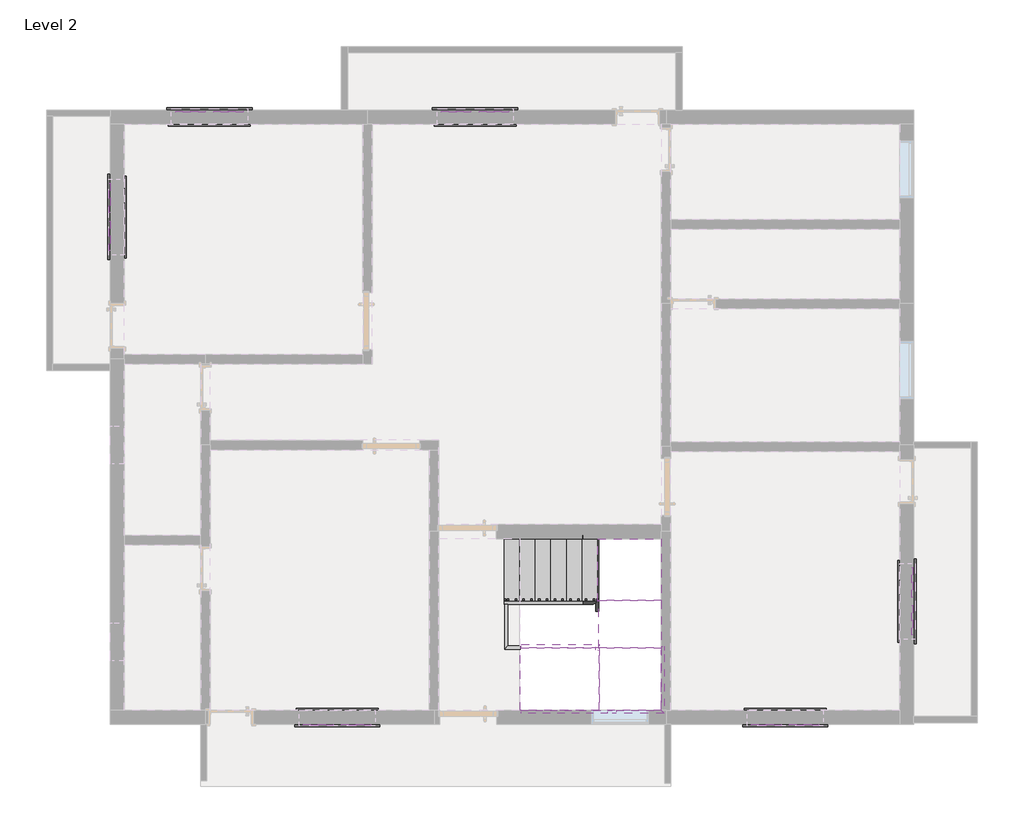
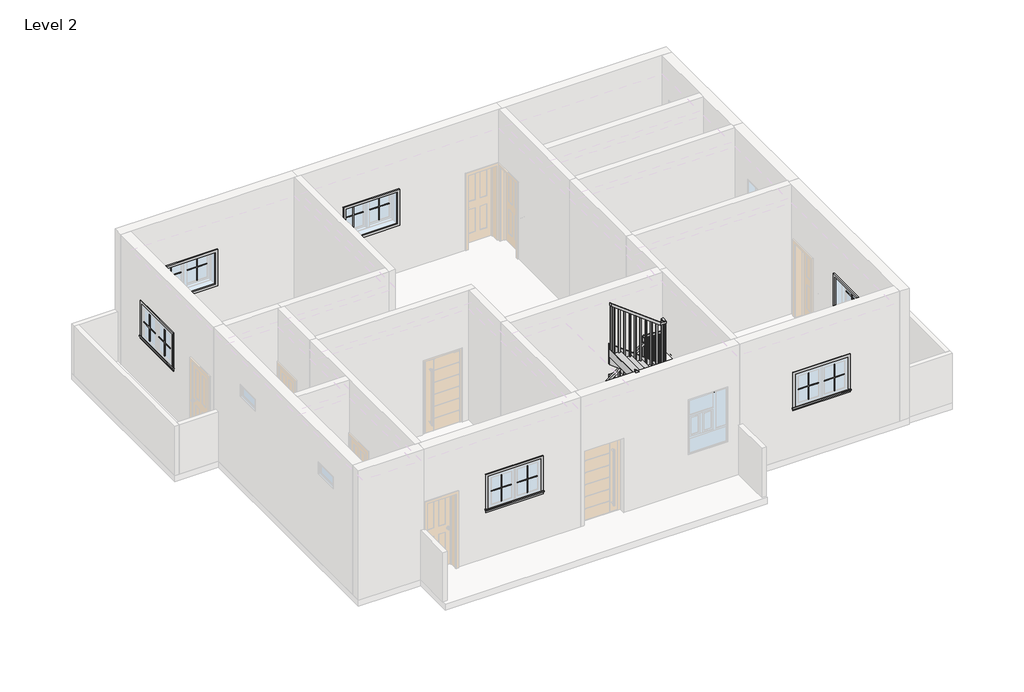
# One storey, part 3 of 3: 24 proxies, 11 members, 3 stair flights, 2 railings, 2 slabs.
"""IFC4 building model written with IfcOpenShell, lengths in millimetres."""

from ifc_helpers import new_model, si_unit, frame, origin, place, context, project, spatial, polyline, outline, extrude, faceted_brep, transform, mapped, element, save
from components import m_muntin_pattern_2x2_m_muntin_pattern_2x2_8d9e5da3, m_muntin_pattern_2x2_m_muntin_pattern_2x2_32a0f80e, m_trim_window_exterior_flat_with_sill_3a557199, m_trim_window_interior_flat_picture_frame_580345df, non_monolithic_landing_c08c66cc, non_monolithic_landing_bd582a30, stair_flight_50mm_tread_13mm_riser_0f073b0c, stair_flight_50mm_tread_13mm_riser_a88b1a6b, stair_flight_50mm_tread_13mm_riser_70c7a40c

model = new_model("IFC4")

# Units and contexts
model_context = context("Model", 3, world=origin())
ifc_project = project(units=[si_unit("LENGTHUNIT", "METRE", prefix="MILLI")], contexts=[model_context])

# Site, building, storey
site = spatial("IfcSite", under=ifc_project)
building = spatial("IfcBuilding", under=site)
storey = spatial("IfcBuildingStorey", under=building, Name="Level 2", Elevation=3200.4)

# Proxies
placement = place(None, origin())
m_muntin_pattern_2x2_m_muntin_pattern_2x2_shape = m_muntin_pattern_2x2_m_muntin_pattern_2x2_8d9e5da3(model_context)
element("IfcBuildingElementProxy", 1, Name="M_Muntin Pattern_2x2 : M_Muntin Pattern_2x2", ObjectType="M_Muntin Pattern_2x2 : M_Muntin Pattern_2x2", at=placement, inside=storey, context=model_context, shape_type="MappedRepresentation", body=[
    mapped(m_muntin_pattern_2x2_m_muntin_pattern_2x2_shape, transform((-14356.7669909, -4470.2368509, 4489.45), x_axis=(-1.0, 0.0, 0.0), y_axis=(0.0, -1.0, 0.0), z_axis=(0.0, 0.0, 1.0))),
])
element("IfcBuildingElementProxy", 2, Name="M_Muntin Pattern_2x2 : M_Muntin Pattern_2x2", ObjectType="M_Muntin Pattern_2x2 : M_Muntin Pattern_2x2", at=placement, inside=storey, context=model_context, shape_type="MappedRepresentation", body=[
    mapped(m_muntin_pattern_2x2_m_muntin_pattern_2x2_shape, transform((-17007.0919909, 5340.5131491, 4489.45), x_axis=(1.0, 0.0, 0.0), y_axis=(0.0, 1.0, 0.0), z_axis=(0.0, 0.0, 1.0))),
])
element("IfcBuildingElementProxy", 3, Name="M_Muntin Pattern_2x2 : M_Muntin Pattern_2x2", ObjectType="M_Muntin Pattern_2x2 : M_Muntin Pattern_2x2", at=placement, inside=storey, context=model_context, shape_type="MappedRepresentation", body=[
    mapped(m_muntin_pattern_2x2_m_muntin_pattern_2x2_shape, transform((-18281.8544909, 3334.7006491, 4489.45), x_axis=(0.0, 1.0, 0.0), y_axis=(-1.0, 0.0, 0.0), z_axis=(0.0, 0.0, 1.0))),
])
element("IfcBuildingElementProxy", 4, Name="M_Muntin Pattern_2x2 : M_Muntin Pattern_2x2", ObjectType="M_Muntin Pattern_2x2 : M_Muntin Pattern_2x2", at=placement, inside=storey, context=model_context, shape_type="MappedRepresentation", body=[
    mapped(m_muntin_pattern_2x2_m_muntin_pattern_2x2_shape, transform((-12757.3544909, 5340.5131491, 4489.45), x_axis=(1.0, 0.0, 0.0), y_axis=(0.0, 1.0, 0.0), z_axis=(0.0, 0.0, 1.0))),
])
element("IfcBuildingElementProxy", 5, Name="M_Muntin Pattern_2x2 : M_Muntin Pattern_2x2", ObjectType="M_Muntin Pattern_2x2 : M_Muntin Pattern_2x2", at=placement, inside=storey, context=model_context, shape_type="MappedRepresentation", body=[
    mapped(m_muntin_pattern_2x2_m_muntin_pattern_2x2_shape, transform((-5448.5044909, -2207.2493509, 4489.45), x_axis=(0.0, -1.0, 0.0), y_axis=(1.0, 0.0, 0.0), z_axis=(0.0, 0.0, 1.0))),
])
element("IfcBuildingElementProxy", 6, Name="M_Muntin Pattern_2x2 : M_Muntin Pattern_2x2", ObjectType="M_Muntin Pattern_2x2 : M_Muntin Pattern_2x2", at=placement, inside=storey, context=model_context, shape_type="MappedRepresentation", body=[
    mapped(m_muntin_pattern_2x2_m_muntin_pattern_2x2_shape, transform((-7193.1669909, -4470.2368509, 4489.45), x_axis=(-1.0, 0.0, 0.0), y_axis=(0.0, -1.0, 0.0), z_axis=(0.0, 0.0, 1.0))),
])
m_muntin_pattern_2x2_m_muntin_pattern_2x2_2_shape = m_muntin_pattern_2x2_m_muntin_pattern_2x2_32a0f80e(model_context)
element("IfcBuildingElementProxy", 7, Name="M_Muntin Pattern_2x2 : M_Muntin Pattern_2x2", ObjectType="M_Muntin Pattern_2x2 : M_Muntin Pattern_2x2", at=placement, inside=storey, context=model_context, shape_type="MappedRepresentation", body=[
    mapped(m_muntin_pattern_2x2_m_muntin_pattern_2x2_2_shape, transform((-14963.1919909, -4470.2368509, 4489.45), x_axis=(1.0, 0.0, 0.0), y_axis=(0.0, 1.0, 0.0), z_axis=(0.0, 0.0, 1.0))),
])
element("IfcBuildingElementProxy", 8, Name="M_Muntin Pattern_2x2 : M_Muntin Pattern_2x2", ObjectType="M_Muntin Pattern_2x2 : M_Muntin Pattern_2x2", at=placement, inside=storey, context=model_context, shape_type="MappedRepresentation", body=[
    mapped(m_muntin_pattern_2x2_m_muntin_pattern_2x2_2_shape, transform((-16400.6669909, 5340.5131491, 4489.45), x_axis=(-1.0, 0.0, 0.0), y_axis=(0.0, -1.0, 0.0), z_axis=(0.0, 0.0, 1.0))),
])
element("IfcBuildingElementProxy", 9, Name="M_Muntin Pattern_2x2 : M_Muntin Pattern_2x2", ObjectType="M_Muntin Pattern_2x2 : M_Muntin Pattern_2x2", at=placement, inside=storey, context=model_context, shape_type="MappedRepresentation", body=[
    mapped(m_muntin_pattern_2x2_m_muntin_pattern_2x2_2_shape, transform((-18281.8544909, 3941.1256491, 4489.45), x_axis=(0.0, -1.0, 0.0), y_axis=(1.0, 0.0, 0.0), z_axis=(0.0, 0.0, 1.0))),
])
element("IfcBuildingElementProxy", 10, Name="M_Muntin Pattern_2x2 : M_Muntin Pattern_2x2", ObjectType="M_Muntin Pattern_2x2 : M_Muntin Pattern_2x2", at=placement, inside=storey, context=model_context, shape_type="MappedRepresentation", body=[
    mapped(m_muntin_pattern_2x2_m_muntin_pattern_2x2_2_shape, transform((-12150.9294909, 5340.5131491, 4489.45), x_axis=(-1.0, 0.0, 0.0), y_axis=(0.0, -1.0, 0.0), z_axis=(0.0, 0.0, 1.0))),
])
element("IfcBuildingElementProxy", 11, Name="M_Muntin Pattern_2x2 : M_Muntin Pattern_2x2", ObjectType="M_Muntin Pattern_2x2 : M_Muntin Pattern_2x2", at=placement, inside=storey, context=model_context, shape_type="MappedRepresentation", body=[
    mapped(m_muntin_pattern_2x2_m_muntin_pattern_2x2_2_shape, transform((-5448.5044909, -2813.6743509, 4489.45), x_axis=(0.0, 1.0, 0.0), y_axis=(-1.0, 0.0, 0.0), z_axis=(0.0, 0.0, 1.0))),
])
element("IfcBuildingElementProxy", 12, Name="M_Muntin Pattern_2x2 : M_Muntin Pattern_2x2", ObjectType="M_Muntin Pattern_2x2 : M_Muntin Pattern_2x2", at=placement, inside=storey, context=model_context, shape_type="MappedRepresentation", body=[
    mapped(m_muntin_pattern_2x2_m_muntin_pattern_2x2_2_shape, transform((-7799.5919909, -4470.2368509, 4489.45), x_axis=(1.0, 0.0, 0.0), y_axis=(0.0, 1.0, 0.0), z_axis=(0.0, 0.0, 1.0))),
])
m_trim_window_exterior_flat_with_sill_shape = m_trim_window_exterior_flat_with_sill_3a557199(model_context)
element("IfcBuildingElementProxy", 13, Name="M_Trim-Window-Exterior-Flat : with Sill", ObjectType="M_Trim-Window-Exterior-Flat : with Sill", at=placement, inside=storey, context=model_context, shape_type="MappedRepresentation", body=[
    mapped(m_trim_window_exterior_flat_with_sill_shape, transform((-14659.9794909, -4479.7618509, 5219.6), x_axis=(1.0, 0.0, 0.0), y_axis=(0.0, 0.0, 1.0), z_axis=(0.0, -1.0, 0.0))),
])
element("IfcBuildingElementProxy", 14, Name="M_Trim-Window-Exterior-Flat : with Sill", ObjectType="M_Trim-Window-Exterior-Flat : with Sill", at=placement, inside=storey, context=model_context, shape_type="MappedRepresentation", body=[
    mapped(m_trim_window_exterior_flat_with_sill_shape, transform((-16703.8794909, 5350.0381491, 5219.6), x_axis=(-1.0, 0.0, 0.0), y_axis=(0.0, 0.0, 1.0), z_axis=(0.0, 1.0, 0.0))),
])
element("IfcBuildingElementProxy", 15, Name="M_Trim-Window-Exterior-Flat : with Sill", ObjectType="M_Trim-Window-Exterior-Flat : with Sill", at=placement, inside=storey, context=model_context, shape_type="MappedRepresentation", body=[
    mapped(m_trim_window_exterior_flat_with_sill_shape, transform((-18291.3794909, 3637.9131491, 5219.6), x_axis=(0.0, -1.0, 0.0), y_axis=(0.0, 0.0, 1.0), z_axis=(-1.0, 0.0, 0.0))),
])
element("IfcBuildingElementProxy", 16, Name="M_Trim-Window-Exterior-Flat : with Sill", ObjectType="M_Trim-Window-Exterior-Flat : with Sill", at=placement, inside=storey, context=model_context, shape_type="MappedRepresentation", body=[
    mapped(m_trim_window_exterior_flat_with_sill_shape, transform((-12454.1419909, 5350.0381491, 5219.6), x_axis=(-1.0, 0.0, 0.0), y_axis=(0.0, 0.0, 1.0), z_axis=(0.0, 1.0, 0.0))),
])
element("IfcBuildingElementProxy", 17, Name="M_Trim-Window-Exterior-Flat : with Sill", ObjectType="M_Trim-Window-Exterior-Flat : with Sill", at=placement, inside=storey, context=model_context, shape_type="MappedRepresentation", body=[
    mapped(m_trim_window_exterior_flat_with_sill_shape, transform((-5438.9794909, -2510.4618509, 5219.6), x_axis=(0.0, 1.0, 0.0), y_axis=(0.0, 0.0, 1.0), z_axis=(1.0, 0.0, 0.0))),
])
element("IfcBuildingElementProxy", 18, Name="M_Trim-Window-Exterior-Flat : with Sill", ObjectType="M_Trim-Window-Exterior-Flat : with Sill", at=placement, inside=storey, context=model_context, shape_type="MappedRepresentation", body=[
    mapped(m_trim_window_exterior_flat_with_sill_shape, transform((-7496.3794909, -4479.7618509, 5219.6), x_axis=(1.0, 0.0, 0.0), y_axis=(0.0, 0.0, 1.0), z_axis=(0.0, -1.0, 0.0))),
])
m_trim_window_interior_flat_picture_frame_shape = m_trim_window_interior_flat_picture_frame_580345df(model_context)
element("IfcBuildingElementProxy", 19, Name="M_Trim-Window-Interior-Flat : Picture Frame", ObjectType="M_Trim-Window-Interior-Flat : Picture Frame", at=placement, inside=storey, context=model_context, shape_type="MappedRepresentation", body=[
    mapped(m_trim_window_interior_flat_picture_frame_shape, transform((-14659.9794909, -4251.1618509, 5219.6), x_axis=(-1.0, 0.0, 0.0), y_axis=(0.0, 0.0, 1.0), z_axis=(0.0, 1.0, 0.0))),
])
element("IfcBuildingElementProxy", 20, Name="M_Trim-Window-Interior-Flat : Picture Frame", ObjectType="M_Trim-Window-Interior-Flat : Picture Frame", at=placement, inside=storey, context=model_context, shape_type="MappedRepresentation", body=[
    mapped(m_trim_window_interior_flat_picture_frame_shape, transform((-16703.8794909, 5121.4381491, 5219.6), x_axis=(1.0, 0.0, 0.0), y_axis=(0.0, 0.0, 1.0), z_axis=(0.0, -1.0, 0.0))),
])
element("IfcBuildingElementProxy", 21, Name="M_Trim-Window-Interior-Flat : Picture Frame", ObjectType="M_Trim-Window-Interior-Flat : Picture Frame", at=placement, inside=storey, context=model_context, shape_type="MappedRepresentation", body=[
    mapped(m_trim_window_interior_flat_picture_frame_shape, transform((-18062.7794909, 3637.9131491, 5219.6), x_axis=(0.0, 1.0, 0.0), y_axis=(0.0, 0.0, 1.0), z_axis=(1.0, 0.0, 0.0))),
])
element("IfcBuildingElementProxy", 22, Name="M_Trim-Window-Interior-Flat : Picture Frame", ObjectType="M_Trim-Window-Interior-Flat : Picture Frame", at=placement, inside=storey, context=model_context, shape_type="MappedRepresentation", body=[
    mapped(m_trim_window_interior_flat_picture_frame_shape, transform((-12454.1419909, 5121.4381491, 5219.6), x_axis=(1.0, 0.0, 0.0), y_axis=(0.0, 0.0, 1.0), z_axis=(0.0, -1.0, 0.0))),
])
element("IfcBuildingElementProxy", 23, Name="M_Trim-Window-Interior-Flat : Picture Frame", ObjectType="M_Trim-Window-Interior-Flat : Picture Frame", at=placement, inside=storey, context=model_context, shape_type="MappedRepresentation", body=[
    mapped(m_trim_window_interior_flat_picture_frame_shape, transform((-5667.5794909, -2510.4618509, 5219.6), x_axis=(0.0, -1.0, 0.0), y_axis=(0.0, 0.0, 1.0), z_axis=(-1.0, 0.0, 0.0))),
])
element("IfcBuildingElementProxy", 24, Name="M_Trim-Window-Interior-Flat : Picture Frame", ObjectType="M_Trim-Window-Interior-Flat : Picture Frame", at=placement, inside=storey, context=model_context, shape_type="MappedRepresentation", body=[
    mapped(m_trim_window_interior_flat_picture_frame_shape, transform((-7496.3794909, -4251.1618509, 5219.6), x_axis=(-1.0, 0.0, 0.0), y_axis=(0.0, 0.0, 1.0), z_axis=(0.0, 1.0, 0.0))),
])

# Members
element("IfcMember", 25, ObjectType="Stringer - 50mm Width", at=placement, inside=storey, context=model_context, shape_type="SweptSolid", body=[
    extrude(outline(polyline([(3453.9429417, -11992.1794909), (3200.4, -11992.1794909), (3200.4, -11663.9259909), (4168.2117647, -10378.7116427), (4568.2117647, -10512.4761733), (3453.9429417, -11992.1794909)])), frame((0.0, -1507.9618509, 0.0), z_axis=(0.0, 1.0, 0.0), x_axis=(0.0, 0.0, 1.0)), (0.0, 0.0, 1.0), 50.0),
])
element("IfcMember", 26, ObjectType="Stringer - 50mm Width", at=placement, inside=storey, context=model_context, shape_type="Brep", body=[
    faceted_brep([(-11992.1794909, -2557.9876321, 3200.4), (-11992.1794909, -2507.9876321, 3200.4), (-11663.9259909, -2507.9876321, 3200.4), (-11663.9259909, -2557.9876321, 3200.4), (-11992.1794909, -2557.9876321, 3453.9429417), (-10569.4898929, -2557.9876321, 4024.549009), (-10569.4898929, -2557.9876321, 4525.2784216), (-10492.1794909, -2507.9876321, 4082.7664703), (-10492.1794909, -2507.9876321, 4568.2117647), (-10512.4761733, -2521.1143795, 4568.2117647), (-11992.1794909, -2507.9876321, 3453.9429417), (-10512.4761733, -2507.9876321, 4568.2117647)], [[[0, 1, 2, 3]], [[4, 0, 3, 5, 6]], [[6, 5, 7, 8, 9]], [[2, 7, 5, 3]], [[1, 10, 11, 8, 7, 2]], [[11, 9, 8]], [[10, 4, 6, 9, 11]], [[4, 10, 1, 0]]]),
])
element("IfcMember", 27, ObjectType="Stringer - 50mm Width", at=placement, inside=storey, context=model_context, shape_type="SweptSolid", body=[
    extrude(outline(polyline([(-2228.2651685, 4568.2117647), (-2362.029699, 4168.2117647), (-3362.029699, 4921.2470588), (-3228.2651685, 5321.2470588), (-2228.2651685, 4568.2117647)])), frame((-9477.5794909, 0.0, 0.0), z_axis=(1.0, 0.0, 0.0), x_axis=(0.0, 1.0, 0.0)), (0.0, 0.0, 1.0), 50.0),
])
element("IfcMember", 28, ObjectType="Stringer - 50mm Width", at=placement, inside=storey, context=model_context, shape_type="Brep", body=[
    faceted_brep([(-10527.6052721, -3234.9066499, 5321.2470588), (-10527.6052721, -3234.9066499, 4825.5189161), (-10477.6052721, -3248.5618509, 4835.8017644), (-10477.6052721, -3248.5618509, 5321.2470588), (-10477.6052721, -3228.2651685, 5321.2470588), (-10527.6052721, -3228.2651685, 5321.2470588), (-10477.6052721, -2498.5618509, 4771.7547064), (-10527.6052721, -2530.8990259, 4796.1057405), (-10477.6052721, -2498.5618509, 4271.0252938), (-10527.6052721, -2530.8990259, 4295.3763279)], [[[0, 1, 2, 3]], [[4, 5, 0, 3]], [[6, 7, 5, 4]], [[7, 6, 8, 9]], [[7, 9, 1, 0, 5]], [[8, 6, 4, 3, 2]], [[9, 8, 2, 1]]]),
])
element("IfcMember", 29, ObjectType="Stringer - 50mm Width", at=placement, inside=storey, context=model_context, shape_type="Brep", body=[
    faceted_brep([(-9477.5794909, -2228.2651685, 4568.2117647), (-9427.5794909, -2228.2651685, 4568.2117647), (-9427.5794909, -1457.9618509, 4568.2117647), (-9477.5794909, -1507.9618509, 4568.2117647), (-9477.5794909, -2362.029699, 4168.2117647), (-9477.5794909, -1507.9618509, 4168.2117647), (-9427.5794909, -2362.029699, 4168.2117647), (-9427.5794909, -1457.9618509, 4168.2117647)], [[[0, 1, 2, 3]], [[4, 0, 3, 5]], [[6, 4, 5, 7]], [[1, 6, 7, 2]], [[1, 0, 4, 6]], [[2, 7, 5, 3]]]),
])
element("IfcMember", 30, ObjectType="Stringer - 50mm Width", at=placement, inside=storey, context=model_context, shape_type="Brep", body=[
    faceted_brep([(-9477.5794909, -1507.9618509, 4568.2117647), (-9427.5794909, -1457.9618509, 4568.2117647), (-10512.4761733, -1457.9618509, 4568.2117647), (-10512.4761733, -1507.9618509, 4568.2117647), (-9477.5794909, -1507.9618509, 4168.2117647), (-10378.7116427, -1507.9618509, 4168.2117647), (-9427.5794909, -1457.9618509, 4168.2117647), (-10378.7116427, -1457.9618509, 4168.2117647)], [[[0, 1, 2, 3]], [[4, 0, 3, 5]], [[6, 4, 5, 7]], [[1, 6, 7, 2]], [[1, 0, 4, 6]], [[2, 7, 5, 3]]]),
])
element("IfcMember", 31, ObjectType="Stringer - 50mm Width", at=placement, inside=storey, context=model_context, shape_type="SweptSolid", body=[
    extrude(outline(polyline([(4921.2470588, -10331.6473391), (5321.2470588, -10197.8828085), (6466.0841182, -11718.1794909), (5965.3547056, -11718.1794909), (4921.2470588, -10331.6473391)])), frame((0.0, -4301.1618509, 0.0), z_axis=(0.0, 1.0, 0.0), x_axis=(0.0, 0.0, 1.0)), (0.0, 0.0, 1.0), 50.0),
])
element("IfcMember", 32, ObjectType="Stringer - 50mm Width", at=placement, inside=storey, context=model_context, shape_type="SweptSolid", body=[
    extrude(outline(polyline([(5024.0605879, -10468.1794909), (5524.7900005, -10468.1794909), (6466.0841182, -11718.1794909), (5965.3547056, -11718.1794909), (5024.0605879, -10468.1794909)])), frame((0.0, -3251.1360696, 0.0), z_axis=(0.0, 1.0, 0.0), x_axis=(0.0, 0.0, 1.0)), (0.0, 0.0, 1.0), 50.0),
])
element("IfcMember", 33, ObjectType="Stringer - 50mm Width", at=placement, inside=storey, context=model_context, shape_type="Brep", body=[
    faceted_brep([(-10197.8828085, -4251.1618509, 5321.2470588), (-10197.8828085, -4301.1618509, 5321.2470588), (-9427.5794909, -4301.1618509, 5321.2470588), (-9477.5794909, -4251.1618509, 5321.2470588), (-10331.6473391, -4251.1618509, 4921.2470588), (-9477.5794909, -4251.1618509, 4921.2470588), (-10331.6473391, -4301.1618509, 4921.2470588), (-9427.5794909, -4301.1618509, 4921.2470588)], [[[0, 1, 2, 3]], [[4, 0, 3, 5]], [[6, 4, 5, 7]], [[1, 6, 7, 2]], [[1, 0, 4, 6]], [[2, 7, 5, 3]]]),
])
element("IfcMember", 34, ObjectType="Stringer - 50mm Width", at=placement, inside=storey, context=model_context, shape_type="Brep", body=[
    faceted_brep([(-9477.5794909, -4251.1618509, 5321.2470588), (-9427.5794909, -4301.1618509, 5321.2470588), (-9427.5794909, -3228.2651685, 5321.2470588), (-9477.5794909, -3228.2651685, 5321.2470588), (-9477.5794909, -4251.1618509, 4921.2470588), (-9477.5794909, -3362.029699, 4921.2470588), (-9427.5794909, -4301.1618509, 4921.2470588), (-9427.5794909, -3362.029699, 4921.2470588)], [[[0, 1, 2, 3]], [[4, 0, 3, 5]], [[6, 4, 5, 7]], [[1, 6, 7, 2]], [[1, 0, 4, 6]], [[2, 7, 5, 3]]]),
])
element("IfcMember", 35, ObjectType="Stringer - 50mm Width", at=placement, inside=storey, context=model_context, shape_type="SweptSolid", body=[
    extrude(outline(polyline([(-10527.6052721, -3286.7377652), (-10527.6052721, -3234.9066499), (-10468.1794909, -3251.1360696), (-10468.1794909, -3302.9671849), (-10527.6052721, -3286.7377652)])), frame((0.0, 0.0, 4921.2470588), z_axis=(0.0, 0.0, 1.0), x_axis=(1.0, 0.0, 0.0)), (0.0, 0.0, 1.0), 400.0),
])

# Railings
element("IfcRailing", 36, ObjectType="1100mm", at=placement, inside=storey, context=model_context, shape_type="SolidModel", body=[
    faceted_brep([(-11992.1794909, -2457.5876321, 4488.6588235), (-11992.1794909, -2457.5876321, 4426.067647), (-11992.1794909, -2507.5876321, 4426.067647), (-11992.1794909, -2507.5876321, 4488.6588235), (-10506.1686883, -2457.5876321, 5607.6774053), (-10493.1861187, -2507.5876321, 5617.4537384), (-10475.1839648, -2507.5876321, 5568.4188191), (-10488.1665344, -2457.5876321, 5558.642486)], [[[0, 1, 2, 3]], [[4, 5, 6, 7]], [[1, 0, 4, 7]], [[2, 1, 7, 6]], [[3, 2, 6, 5]], [[0, 3, 5, 4]]]),
    faceted_brep([(-10507.8033465, -2458.0701724, 5618.2117647), (-10492.6871017, -2448.2938394, 5568.2117647), (-10476.4352157, -2497.3287587, 5568.2117647), (-10491.5514605, -2507.1050918, 5618.2117647), (-10486.7741604, -2444.469683, 5618.2117647), (-10459.6209288, -2486.4542279, 5618.2117647), (-10417.6363839, -2459.3009964, 5568.2117647), (-10444.7896154, -2417.3164514, 5568.2117647)], [[[0, 1, 2, 3]], [[4, 5, 6, 7]], [[1, 0, 4, 7]], [[2, 1, 7, 6]], [[3, 2, 6, 5]], [[0, 3, 5, 4]]]),
    faceted_brep([(-10486.7741604, -2444.469683, 5618.2117647), (-10444.7896154, -2417.3164514, 5568.2117647), (-10417.6363839, -2459.3009964, 5568.2117647), (-10459.6209288, -2486.4542279, 5618.2117647), (-10486.7741604, -2444.469683, 5743.724782), (-10459.6209288, -2486.4542279, 5722.7833848), (-10417.6363839, -2459.3009964, 5736.3270973), (-10444.7896154, -2417.3164514, 5757.2684945)], [[[0, 1, 2, 3]], [[4, 5, 6, 7]], [[1, 0, 4, 7]], [[2, 1, 7, 6]], [[3, 2, 6, 5]], [[0, 3, 5, 4]]]),
    faceted_brep([(-10427.2052721, -2426.8853397, 5752.4956456), (-10427.2052721, -2476.8853397, 5727.5562337), (-10477.2052721, -2476.8853397, 5727.5562337), (-10477.2052721, -2426.8853397, 5752.4956456), (-10427.2052721, -3176.5360696, 6317.0091035), (-10427.2052721, -3226.5360696, 6292.0696916), (-10477.2052721, -3226.5360696, 6292.0696916), (-10477.2052721, -3176.5360696, 6317.0091035), (-10427.2052721, -3176.5360696, 6622.7802613), (-10427.2052721, -3226.5360696, 6572.7802613), (-10477.2052721, -3226.5360696, 6572.7802613), (-10477.2052721, -3176.5360696, 6622.7802613), (-10427.2052721, -3301.5360696, 6622.7802613), (-10427.2052721, -3301.5360696, 6572.7802613), (-10477.2052721, -3251.5360696, 6572.7802613), (-10477.2052721, -3251.5360696, 6622.7802613), (-10552.2052721, -3301.5360696, 6622.7802613), (-10568.9258385, -3301.5360696, 6572.7802613), (-10568.9258385, -3251.5360696, 6572.7802613), (-10552.2052721, -3251.5360696, 6622.7802613), (-11718.1794909, -3301.5360696, 7500.8), (-11718.1794909, -3251.5360696, 7500.8), (-11718.1794909, -3251.5360696, 7438.2088234), (-11718.1794909, -3301.5360696, 7438.2088234)], [[[0, 1, 2, 3]], [[1, 0, 4, 5]], [[2, 1, 5, 6]], [[3, 2, 6, 7]], [[0, 3, 7, 4]], [[5, 4, 8, 9]], [[6, 5, 9, 10]], [[7, 6, 10, 11]], [[4, 7, 11, 8]], [[9, 8, 12, 13]], [[10, 9, 13, 14]], [[11, 10, 14, 15]], [[8, 11, 15, 12]], [[13, 12, 16, 17]], [[14, 13, 17, 18]], [[15, 14, 18, 19]], [[12, 15, 19, 16]], [[20, 21, 22, 23]], [[17, 16, 20, 23]], [[18, 17, 23, 22]], [[19, 18, 22, 21]], [[16, 19, 21, 20]]]),
    extrude(outline(polyline([(6212.5411765, -11627.2052721), (7369.7020258, -11627.2052721), (7388.5279082, -11652.2052721), (6212.5411765, -11652.2052721), (6212.5411765, -11627.2052721)])), frame((0.0, -3289.0360696, 0.0), z_axis=(0.0, 1.0, 0.0), x_axis=(0.0, 0.0, 1.0)), (0.0, 0.0, 1.0), 25.0),
    extrude(outline(polyline([(6212.5411765, -11502.2052721), (7275.5726141, -11502.2052721), (7294.3984964, -11527.2052721), (6212.5411765, -11527.2052721), (6212.5411765, -11502.2052721)])), frame((0.0, -3289.0360696, 0.0), z_axis=(0.0, 1.0, 0.0), x_axis=(0.0, 0.0, 1.0)), (0.0, 0.0, 1.0), 25.0),
    extrude(outline(polyline([(6024.2823529, -11377.2052721), (7181.4432023, -11377.2052721), (7200.2690847, -11402.2052721), (6024.2823529, -11402.2052721), (6024.2823529, -11377.2052721)])), frame((0.0, -3289.0360696, 0.0), z_axis=(0.0, 1.0, 0.0), x_axis=(0.0, 0.0, 1.0)), (0.0, 0.0, 1.0), 25.0),
    extrude(outline(polyline([(6024.2823529, -11252.2052721), (7087.3137906, -11252.2052721), (7106.1396729, -11277.2052721), (6024.2823529, -11277.2052721), (6024.2823529, -11252.2052721)])), frame((0.0, -3289.0360696, 0.0), z_axis=(0.0, 1.0, 0.0), x_axis=(0.0, 0.0, 1.0)), (0.0, 0.0, 1.0), 25.0),
    extrude(outline(polyline([(5836.0235294, -11127.2052721), (6993.1843788, -11127.2052721), (7012.0102611, -11152.2052721), (5836.0235294, -11152.2052721), (5836.0235294, -11127.2052721)])), frame((0.0, -3289.0360696, 0.0), z_axis=(0.0, 1.0, 0.0), x_axis=(0.0, 0.0, 1.0)), (0.0, 0.0, 1.0), 25.0),
    extrude(outline(polyline([(5836.0235294, -11002.2052721), (6899.054967, -11002.2052721), (6917.8808494, -11027.2052721), (5836.0235294, -11027.2052721), (5836.0235294, -11002.2052721)])), frame((0.0, -3289.0360696, 0.0), z_axis=(0.0, 1.0, 0.0), x_axis=(0.0, 0.0, 1.0)), (0.0, 0.0, 1.0), 25.0),
    extrude(outline(polyline([(5647.7647059, -10877.2052721), (6804.9255553, -10877.2052721), (6823.7514376, -10902.2052721), (5647.7647059, -10902.2052721), (5647.7647059, -10877.2052721)])), frame((0.0, -3289.0360696, 0.0), z_axis=(0.0, 1.0, 0.0), x_axis=(0.0, 0.0, 1.0)), (0.0, 0.0, 1.0), 25.0),
    extrude(outline(polyline([(5647.7647059, -10752.2052721), (6710.7961435, -10752.2052721), (6729.6220258, -10777.2052721), (5647.7647059, -10777.2052721), (5647.7647059, -10752.2052721)])), frame((0.0, -3289.0360696, 0.0), z_axis=(0.0, 1.0, 0.0), x_axis=(0.0, 0.0, 1.0)), (0.0, 0.0, 1.0), 25.0),
    extrude(outline(polyline([(5459.5058824, -10627.2052721), (6616.6667317, -10627.2052721), (6635.4926141, -10652.2052721), (5459.5058824, -10652.2052721), (5459.5058824, -10627.2052721)])), frame((0.0, -3289.0360696, 0.0), z_axis=(0.0, 1.0, 0.0), x_axis=(0.0, 0.0, 1.0)), (0.0, 0.0, 1.0), 25.0),
    extrude(outline(polyline([(-10502.2052721, -3264.0360696), (-10502.2052721, -3289.0360696), (-10527.2052721, -3289.0360696), (-10527.2052721, -3264.0360696), (-10502.2052721, -3264.0360696)])), frame((0.0, 0.0, 5459.5058824), z_axis=(0.0, 0.0, 1.0), x_axis=(1.0, 0.0, 0.0)), (0.0, 0.0, 1.0), 1113.2743789),
    extrude(outline(polyline([(-10464.7052721, -3251.8853397), (-10439.7052721, -3251.8853397), (-10439.7052721, -3276.8853397), (-10464.7052721, -3276.8853397), (-10464.7052721, -3251.8853397)])), frame((0.0, 0.0, 5271.2470588), z_axis=(0.0, 0.0, 1.0), x_axis=(1.0, 0.0, 0.0)), (0.0, 0.0, 1.0), 1301.5332024),
    extrude(outline(polyline([(-3126.8853397, 6217.0291749), (-3126.8853397, 5082.9882353), (-3151.8853397, 5082.9882353), (-3151.8853397, 6235.8550572), (-3126.8853397, 6217.0291749)])), frame((-10464.7052721, 0.0, 0.0), z_axis=(1.0, 0.0, 0.0), x_axis=(0.0, 1.0, 0.0)), (0.0, 0.0, 1.0), 25.0),
    extrude(outline(polyline([(-3001.8853397, 6122.8997631), (-3001.8853397, 5082.9882353), (-3026.8853397, 5082.9882353), (-3026.8853397, 6141.7256455), (-3001.8853397, 6122.8997631)])), frame((-10464.7052721, 0.0, 0.0), z_axis=(1.0, 0.0, 0.0), x_axis=(0.0, 1.0, 0.0)), (0.0, 0.0, 1.0), 25.0),
    extrude(outline(polyline([(-2876.8853397, 6028.7703513), (-2876.8853397, 4894.7294118), (-2901.8853397, 4894.7294118), (-2901.8853397, 6047.5962337), (-2876.8853397, 6028.7703513)])), frame((-10464.7052721, 0.0, 0.0), z_axis=(1.0, 0.0, 0.0), x_axis=(0.0, 1.0, 0.0)), (0.0, 0.0, 1.0), 25.0),
    extrude(outline(polyline([(-2751.8853397, 5934.6409396), (-2751.8853397, 4894.7294118), (-2776.8853397, 4894.7294118), (-2776.8853397, 5953.4668219), (-2751.8853397, 5934.6409396)])), frame((-10464.7052721, 0.0, 0.0), z_axis=(1.0, 0.0, 0.0), x_axis=(0.0, 1.0, 0.0)), (0.0, 0.0, 1.0), 25.0),
    extrude(outline(polyline([(-2626.8853397, 5840.5115278), (-2626.8853397, 4706.4705882), (-2651.8853397, 4706.4705882), (-2651.8853397, 5859.3374102), (-2626.8853397, 5840.5115278)])), frame((-10464.7052721, 0.0, 0.0), z_axis=(1.0, 0.0, 0.0), x_axis=(0.0, 1.0, 0.0)), (0.0, 0.0, 1.0), 25.0),
    extrude(outline(polyline([(-2501.8853397, 5746.382116), (-2501.8853397, 4706.4705882), (-2526.8853397, 4706.4705882), (-2526.8853397, 5765.2079984), (-2501.8853397, 5746.382116)])), frame((-10464.7052721, 0.0, 0.0), z_axis=(1.0, 0.0, 0.0), x_axis=(0.0, 1.0, 0.0)), (0.0, 0.0, 1.0), 25.0),
    extrude(outline(polyline([(5499.1429411, -10567.1794909), (4329.9529412, -10567.1794909), (4329.9529412, -10542.1794909), (5517.9688234, -10542.1794909), (5499.1429411, -10567.1794909)])), frame((0.0, -2495.0876321, 0.0), z_axis=(0.0, 1.0, 0.0), x_axis=(0.0, 0.0, 1.0)), (0.0, 0.0, 1.0), 25.0),
    extrude(outline(polyline([(5405.0135293, -10692.1794909), (4329.9529412, -10692.1794909), (4329.9529412, -10667.1794909), (5423.8394117, -10667.1794909), (5405.0135293, -10692.1794909)])), frame((0.0, -2495.0876321, 0.0), z_axis=(0.0, 1.0, 0.0), x_axis=(0.0, 0.0, 1.0)), (0.0, 0.0, 1.0), 25.0),
    extrude(outline(polyline([(5310.8841175, -10817.1794909), (4141.6941176, -10817.1794909), (4141.6941176, -10792.1794909), (5329.7099999, -10792.1794909), (5310.8841175, -10817.1794909)])), frame((0.0, -2495.0876321, 0.0), z_axis=(0.0, 1.0, 0.0), x_axis=(0.0, 0.0, 1.0)), (0.0, 0.0, 1.0), 25.0),
    extrude(outline(polyline([(5216.7547058, -10942.1794909), (4141.6941176, -10942.1794909), (4141.6941176, -10917.1794909), (5235.5805881, -10917.1794909), (5216.7547058, -10942.1794909)])), frame((0.0, -2495.0876321, 0.0), z_axis=(0.0, 1.0, 0.0), x_axis=(0.0, 0.0, 1.0)), (0.0, 0.0, 1.0), 25.0),
    extrude(outline(polyline([(5122.625294, -11067.1794909), (3953.4352941, -11067.1794909), (3953.4352941, -11042.1794909), (5141.4511764, -11042.1794909), (5122.625294, -11067.1794909)])), frame((0.0, -2495.0876321, 0.0), z_axis=(0.0, 1.0, 0.0), x_axis=(0.0, 0.0, 1.0)), (0.0, 0.0, 1.0), 25.0),
    extrude(outline(polyline([(5028.4958822, -11192.1794909), (3953.4352941, -11192.1794909), (3953.4352941, -11167.1794909), (5047.3217646, -11167.1794909), (5028.4958822, -11192.1794909)])), frame((0.0, -2495.0876321, 0.0), z_axis=(0.0, 1.0, 0.0), x_axis=(0.0, 0.0, 1.0)), (0.0, 0.0, 1.0), 25.0),
    extrude(outline(polyline([(4934.3664705, -11317.1794909), (3765.1764706, -11317.1794909), (3765.1764706, -11292.1794909), (4953.1923528, -11292.1794909), (4934.3664705, -11317.1794909)])), frame((0.0, -2495.0876321, 0.0), z_axis=(0.0, 1.0, 0.0), x_axis=(0.0, 0.0, 1.0)), (0.0, 0.0, 1.0), 25.0),
    extrude(outline(polyline([(4840.2370587, -11442.1794909), (3765.1764706, -11442.1794909), (3765.1764706, -11417.1794909), (4859.0629411, -11417.1794909), (4840.2370587, -11442.1794909)])), frame((0.0, -2495.0876321, 0.0), z_axis=(0.0, 1.0, 0.0), x_axis=(0.0, 0.0, 1.0)), (0.0, 0.0, 1.0), 25.0),
    extrude(outline(polyline([(4746.107647, -11567.1794909), (3576.9176471, -11567.1794909), (3576.9176471, -11542.1794909), (4764.9335293, -11542.1794909), (4746.107647, -11567.1794909)])), frame((0.0, -2495.0876321, 0.0), z_axis=(0.0, 1.0, 0.0), x_axis=(0.0, 0.0, 1.0)), (0.0, 0.0, 1.0), 25.0),
    extrude(outline(polyline([(4651.9782352, -11692.1794909), (3576.9176471, -11692.1794909), (3576.9176471, -11667.1794909), (4670.8041175, -11667.1794909), (4651.9782352, -11692.1794909)])), frame((0.0, -2495.0876321, 0.0), z_axis=(0.0, 1.0, 0.0), x_axis=(0.0, 0.0, 1.0)), (0.0, 0.0, 1.0), 25.0),
    extrude(outline(polyline([(4557.8488234, -11817.1794909), (3388.6588235, -11817.1794909), (3388.6588235, -11792.1794909), (4576.6747058, -11792.1794909), (4557.8488234, -11817.1794909)])), frame((0.0, -2495.0876321, 0.0), z_axis=(0.0, 1.0, 0.0), x_axis=(0.0, 0.0, 1.0)), (0.0, 0.0, 1.0), 25.0),
    extrude(outline(polyline([(4463.7194117, -11942.1794909), (3388.6588235, -11942.1794909), (3388.6588235, -11917.1794909), (4482.545294, -11917.1794909), (4463.7194117, -11942.1794909)])), frame((0.0, -2495.0876321, 0.0), z_axis=(0.0, 1.0, 0.0), x_axis=(0.0, 0.0, 1.0)), (0.0, 0.0, 1.0), 25.0),
    extrude(outline(polyline([(-10464.7052721, -3264.0360696), (-10439.7052721, -3264.0360696), (-10439.7052721, -3289.0360696), (-10464.7052721, -3289.0360696), (-10464.7052721, -3264.0360696)])), frame((0.0, 0.0, 5271.2470588), z_axis=(0.0, 0.0, 1.0), x_axis=(1.0, 0.0, 0.0)), (0.0, 0.0, 1.0), 1301.5332024),
    extrude(outline(polyline([(-10455.9131005, -2469.1697838), (-10469.4897163, -2448.1775113), (-10448.4974438, -2434.6008955), (-10434.920828, -2455.593168), (-10455.9131005, -2469.1697838)])), frame((0.0, 0.0, 4518.2117647), z_axis=(0.0, 0.0, 1.0), x_axis=(1.0, 0.0, 0.0)), (0.0, 0.0, 1.0), 1050.0),
    extrude(outline(polyline([(5540.5614541, -10512.1774035), (4329.9529412, -10512.1774035), (4329.9529412, -10487.1774035), (5559.3873365, -10487.1774035), (5540.5614541, -10512.1774035)])), frame((0.0, -2495.0876321, 0.0), z_axis=(0.0, 1.0, 0.0), x_axis=(0.0, 0.0, 1.0)), (0.0, 0.0, 1.0), 25.0),
    extrude(outline(polyline([(6212.5411765, -11693.1794909), (7419.3829411, -11693.1794909), (7438.2088234, -11718.1794909), (6212.5411765, -11718.1794909), (6212.5411765, -11693.1794909)])), frame((0.0, -3289.0360696, 0.0), z_axis=(0.0, 1.0, 0.0), x_axis=(0.0, 0.0, 1.0)), (0.0, 0.0, 1.0), 25.0),
    extrude(outline(polyline([(4426.067647, -11992.1794909), (3388.6588235, -11992.1794909), (3388.6588235, -11967.1794909), (4444.8935293, -11967.1794909), (4426.067647, -11992.1794909)])), frame((0.0, -2495.0876321, 0.0), z_axis=(0.0, 1.0, 0.0), x_axis=(0.0, 0.0, 1.0)), (0.0, 0.0, 1.0), 25.0),
])
element("IfcRailing", 37, ObjectType="900mm", at=placement, inside=storey, context=model_context, shape_type="SolidModel", body=[
    faceted_brep([(-11730.6794909, -3276.1360696, 4241.8), (-11730.6794909, -3276.1360696, 4191.8), (-11730.6794909, -3226.1360696, 4191.8), (-11730.6794909, -3226.1360696, 4241.8), (-11984.2794909, -3276.1360696, 4241.8), (-11984.2794909, -3276.1360696, 4191.8), (-11934.2794909, -3226.1360696, 4191.8), (-11934.2794909, -3226.1360696, 4241.8), (-11984.2794909, -2557.9876321, 4241.8), (-11934.2794909, -2557.9876321, 4241.8), (-11934.2794909, -2557.9876321, 4191.8), (-11984.2794909, -2557.9876321, 4191.8)], [[[0, 1, 2, 3]], [[1, 0, 4, 5]], [[2, 1, 5, 6]], [[3, 2, 6, 7]], [[0, 3, 7, 4]], [[8, 9, 10, 11]], [[5, 4, 8, 11]], [[6, 5, 11, 10]], [[7, 6, 10, 9]], [[4, 7, 9, 8]]]),
    extrude(outline(polyline([(-11949.2794909, -2711.1360696), (-11969.2794909, -2711.1360696), (-11969.2794909, -2691.1360696), (-11949.2794909, -2691.1360696), (-11949.2794909, -2711.1360696)])), frame((0.0, 0.0, 3200.4), z_axis=(0.0, 0.0, 1.0), x_axis=(1.0, 0.0, 0.0)), (0.0, 0.0, 1.0), 991.4),
    extrude(outline(polyline([(-11949.2794909, -2986.1360696), (-11969.2794909, -2986.1360696), (-11969.2794909, -2966.1360696), (-11949.2794909, -2966.1360696), (-11949.2794909, -2986.1360696)])), frame((0.0, 0.0, 3200.4), z_axis=(0.0, 0.0, 1.0), x_axis=(1.0, 0.0, 0.0)), (0.0, 0.0, 1.0), 991.4),
    extrude(outline(polyline([(-11949.2794909, -3241.1360696), (-11949.2794909, -3261.1360696), (-11969.2794909, -3261.1360696), (-11969.2794909, -3241.1360696), (-11949.2794909, -3241.1360696)])), frame((0.0, 0.0, 3200.4), z_axis=(0.0, 0.0, 1.0), x_axis=(1.0, 0.0, 0.0)), (0.0, 0.0, 1.0), 991.4),
    extrude(outline(polyline([(-11949.2794909, -2577.9876321), (-11969.2794909, -2577.9876321), (-11969.2794909, -2557.9876321), (-11949.2794909, -2557.9876321), (-11949.2794909, -2577.9876321)])), frame((0.0, 0.0, 3200.4), z_axis=(0.0, 0.0, 1.0), x_axis=(1.0, 0.0, 0.0)), (0.0, 0.0, 1.0), 991.4),
    extrude(outline(polyline([(-11730.6794909, -3241.1360696), (-11730.6794909, -3261.1360696), (-11750.6794909, -3261.1360696), (-11750.6794909, -3241.1360696), (-11730.6794909, -3241.1360696)])), frame((0.0, 0.0, 3200.4), z_axis=(0.0, 0.0, 1.0), x_axis=(1.0, 0.0, 0.0)), (0.0, 0.0, 1.0), 991.4),
])

# Slabs
non_monolithic_landing_shape = non_monolithic_landing_c08c66cc(model_context)
element("IfcSlab", 38, ObjectType="Non-Monolithic Landing", at=placement, inside=storey, context=model_context, shape_type="MappedRepresentation", body=[
    mapped(non_monolithic_landing_shape, transform((0.0, 0.0, 0.0), x_axis=(1.0, 0.0, 0.0), y_axis=(0.0, 1.0, 0.0), z_axis=(0.0, 0.0, 1.0))),
])
non_monolithic_landing_2_shape = non_monolithic_landing_bd582a30(model_context)
element("IfcSlab", 39, ObjectType="Non-Monolithic Landing", at=placement, inside=storey, context=model_context, shape_type="MappedRepresentation", body=[
    mapped(non_monolithic_landing_2_shape, transform((0.0, 0.0, 0.0), x_axis=(1.0, 0.0, 0.0), y_axis=(0.0, 1.0, 0.0), z_axis=(0.0, 0.0, 1.0))),
])

# Stair flights
stair_flight_50mm_tread_13mm_riser_shape = stair_flight_50mm_tread_13mm_riser_0f073b0c(model_context)
element("IfcStairFlight", 40, ObjectType="50mm Tread 13mm Riser", at=placement, inside=storey, context=model_context, shape_type="MappedRepresentation", body=[
    mapped(stair_flight_50mm_tread_13mm_riser_shape, transform((0.0, 0.0, 0.0), x_axis=(1.0, 0.0, 0.0), y_axis=(0.0, 1.0, 0.0), z_axis=(0.0, 0.0, 1.0))),
])
stair_flight_50mm_tread_13mm_riser_2_shape = stair_flight_50mm_tread_13mm_riser_a88b1a6b(model_context)
element("IfcStairFlight", 41, ObjectType="50mm Tread 13mm Riser", at=placement, inside=storey, context=model_context, shape_type="MappedRepresentation", body=[
    mapped(stair_flight_50mm_tread_13mm_riser_2_shape, transform((0.0, 0.0, 0.0), x_axis=(1.0, 0.0, 0.0), y_axis=(0.0, 1.0, 0.0), z_axis=(0.0, 0.0, 1.0))),
])
stair_flight_50mm_tread_13mm_riser_3_shape = stair_flight_50mm_tread_13mm_riser_70c7a40c(model_context)
element("IfcStairFlight", 42, ObjectType="50mm Tread 13mm Riser", at=placement, inside=storey, context=model_context, shape_type="MappedRepresentation", body=[
    mapped(stair_flight_50mm_tread_13mm_riser_3_shape, transform((0.0, 0.0, 0.0), x_axis=(1.0, 0.0, 0.0), y_axis=(0.0, 1.0, 0.0), z_axis=(0.0, 0.0, 1.0))),
])

save(model, "model.ifc")

# Revit data of these elements
# Type "M_Muntin Pattern_2x2 : M_Muntin Pattern_2x2"
#   Width [instance default] = 3' - 11.24409"
#   Thickness = 0' - 0 1/2"
#   Height [instance default] = 3' - 11.24409"
#   Distance = 0' - 0 3/4"
#   Interior Material [instance default] = none
#   Exterior Material [instance default] = none
#   Default Elevation = 0
# Type "M_Trim-Window-Exterior-Flat : with Sill"
#   Trim Width = 0' - 2.3622"
#   Trim Thickness_Picture Frame = 0' - 1.1811"
#   Trim Thickness_with Sill = 0' - 0 3/4"
#   Sill Thickness = 0' - 1.1811"
#   Opening Width [instance default] = 1' - 11.62205"
#   Opening Height [instance default] = 2' - 11.43307"
#   Default Elevation = 3' - 11.24409"
#   Sill = yes
#   Picture Frame = no
#   Trim Material [instance default] = none
# Type "M_Trim-Window-Interior-Flat : Picture Frame"
#   Trim Thickness_Picture Frame = 0' - 1.1811"
#   Trim Width = 0' - 2.3622"
#   Trim Thickness_with Sill = 0' - 0.7874"
#   Sill Thickness = 0' - 1.1811"
#   Opening Width [instance default] = 1' - 11.62205"
#   Opening Height [instance default] = 2' - 11.43307"
#   Default Elevation = 3' - 11.24409"
#   Sill = no
#   Picture Frame = yes
#   Trim Material [instance default] = none
# Type "1100mm"
#   built-in parameter 1008612 = 0.019685 (stored number, unit not read)
#   built-in parameter 1008611 = 0.019685 (stored number, unit not read)
#   built-in parameter 1008609 = 0.902231 (stored number, unit not read)
#   built-in parameter 1008604 = 0.19685 (stored number, unit not read)
#   built-in parameter 1008603 = 0.164042 (stored number, unit not read)
#   Railing Height = 3' - 7.30709"
#   built-in parameter 1008630 = 2
#   built-in parameter 1008610 = 2
#   built-in parameter 1008608 = 1
#   built-in parameter 1008618 = M_Baluster - Square : 25mm
# Type "900mm"
#   built-in parameter 1008612 = 0.019685 (stored number, unit not read)
#   built-in parameter 1008611 = 0.019685 (stored number, unit not read)
#   built-in parameter 1008609 = 0.902231 (stored number, unit not read)
#   built-in parameter 1008604 = 0.19685 (stored number, unit not read)
#   built-in parameter 1008603 = 0.164042 (stored number, unit not read)
#   Railing Height = 3' - 5"
#   built-in parameter 1008630 = 2
#   built-in parameter 1008610 = 2
#   built-in parameter 1008608 = 1
#   built-in parameter 1008618 = M_Baluster - Square : 20mm
# Elements 1, 2, 3, 4, 5, 6, 7, 8, 9, 10, 11, 12 (IfcBuildingElementProxy, "M_Muntin Pattern_2x2 : M_Muntin Pattern_2x2")
#   Width = 1' - 6 5/8"
#   Height = 2' - 1.99606"
#   Interior Material = Wood - Stained
#   Exterior Material = Clad - White
#   Phase Created = New Construction
#   Materials on its faces: "Clad - White", "Wood - Stained"
# Elements 13, 14, 15, 16, 17, 18 (IfcBuildingElementProxy, "M_Trim-Window-Exterior-Flat : with Sill")
#   Opening Width = 4' - 0"
#   Opening Height = 2' - 7.49606"
#   Trim Material = Clad - White
#   Phase Created = New Construction
#   Materials on its faces: "Clad - White"
# Elements 19, 20, 21, 22, 23, 24 (IfcBuildingElementProxy, "M_Trim-Window-Interior-Flat : Picture Frame")
#   Opening Width = 4' - 0"
#   Opening Height = 2' - 7.49606"
#   Trim Material = Wood - Stained
#   Phase Created = New Construction
#   Materials on its faces: "Wood - Stained"
# Elements 25, 26, 27, 28, 29, 30, 31, 32, 33, 34, 35 (IfcMember, "Stringer - 50mm Width")
#   Phase Created = New Construction
# Element 36 (IfcRailing, "1100mm")
#   Phase Created = New Construction
# Element 37 (IfcRailing, "900mm")
#   Phase Created = New Construction
# Elements 38, 39 (IfcSlab, "Non-Monolithic Landing")
#   Phase Created = New Construction
# Elements 40, 41, 42 (IfcStairFlight, "50mm Tread 13mm Riser")
#   Phase Created = New Construction
# Materials
#   "Clad - White": class "Wood", colour RGB 242 242 238, transparency 0, Cost = 0
#   "Wood - Stained": class "Wood", colour RGB 224 178 126, transparency 0, Cost = 0
